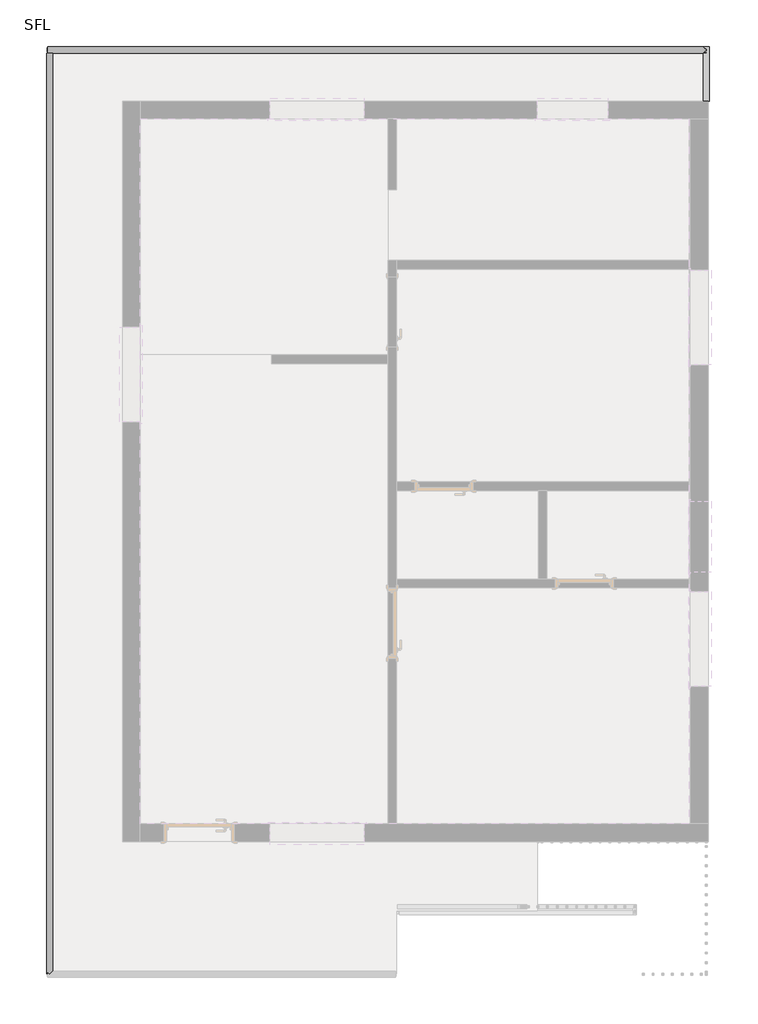
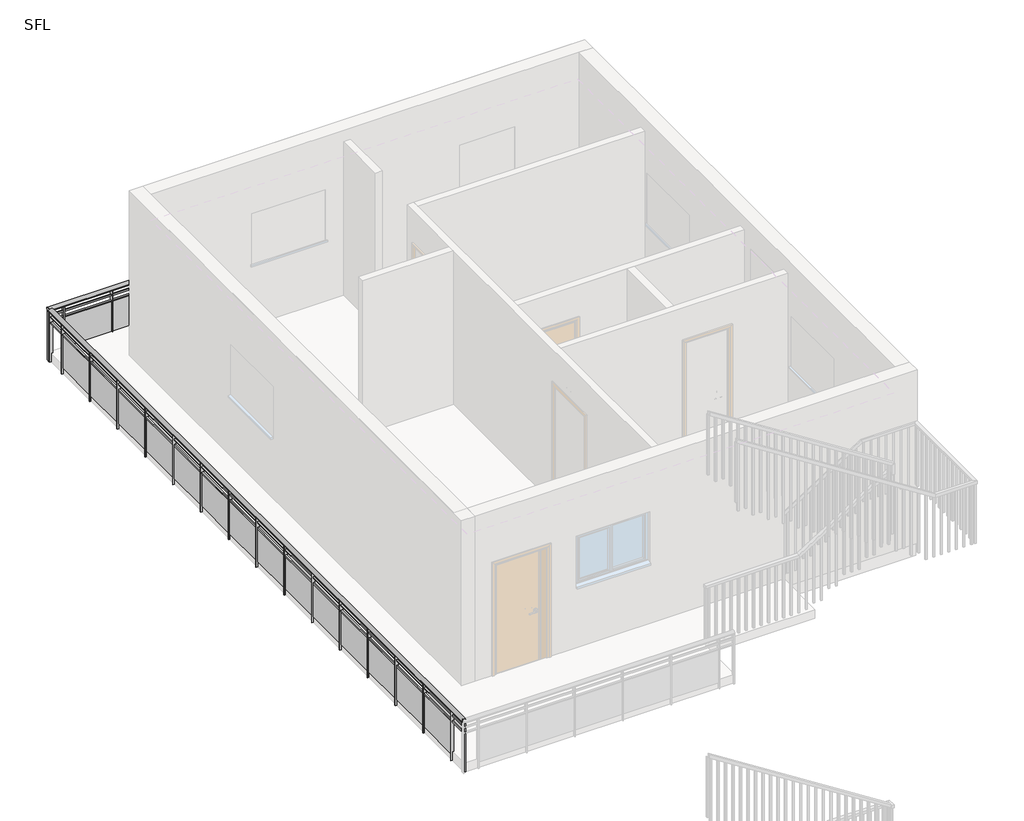
# One storey, part 4 of 4: 3 railings.
"""IFC4 building model written with IfcOpenShell, lengths in millimetres."""

from ifc_helpers import new_model, si_unit, point, frame, origin, place, context, project, spatial, polyline, ellipse_curve, trimmed, outline, extrude, element, save
from ifc_brep_helpers import plane_surface, extruded_surface, advanced_brep

model = new_model("IFC4")

# Units and contexts
model_context = context("Model", 3, world=origin())
ifc_project = project(units=[si_unit("LENGTHUNIT", "METRE", prefix="MILLI")], contexts=[model_context])

# Site, building, storey
site = spatial("IfcSite", under=ifc_project)
building = spatial("IfcBuilding", under=site)
storey = spatial("IfcBuildingStorey", under=building, Name="SFL", Elevation=6583.68)

# Railings
placement = place(None, origin())
element("IfcRailing", 1, ObjectType="Glass_Panel-Bottom_Fill", at=placement, inside=storey, context=model_context, shape_type="SolidModel", body=[
    advanced_brep(
    [(-15004.4132565, 42.847874, 7483.68), (-15004.4132565, -37.152126, 7483.68), (-6495.4132565, 42.847874, 7483.68), (-6495.4132565, -37.152126, 7483.68)],
    [
        (0, 1, ellipse_curve(frame((-15004.4132565, 2.847874, 7483.68), z_axis=(-1.0, 0.0, 0.0), x_axis=(0.0, -1.0, 0.0)), 40.0, 30.0)),
        (1, 0, ellipse_curve(frame((-15004.4132565, 2.847874, 7483.68), z_axis=(-1.0, 0.0, 0.0), x_axis=(0.0, -1.0, 0.0)), 40.0, 30.0)),
        (2, 3, ellipse_curve(frame((-6495.4132565, 2.847874, 7483.68), z_axis=(1.0, 0.0, 0.0), x_axis=(0.0, -1.0, 0.0)), 40.0, 30.0)),
        (3, 2, ellipse_curve(frame((-6495.4132565, 2.847874, 7483.68), z_axis=(1.0, 0.0, 0.0), x_axis=(0.0, -1.0, 0.0)), 40.0, 30.0)),
        (0, 2),
        (3, 1),
    ],
    [
        plane_surface(frame((-15004.4132565, 2.847874, 7483.68), z_axis=(-1.0, 0.0, 0.0), x_axis=(0.0, 1.0, 0.0))),
        plane_surface(frame((-6495.4132565, 2.847874, 7483.68), z_axis=(1.0, 0.0, 0.0), x_axis=(0.0, 1.0, 0.0))),
        extruded_surface(trimmed(ellipse_curve(frame((-6495.4132565, 2.847874, 7483.68), z_axis=(-1.0, 0.0, 0.0), x_axis=(0.0, -1.0, 0.0)), 40.0, 30.0), [point((-6495.4132565, 42.847874, 7483.68))], [point((-6495.4132565, -37.152126, 7483.68))], True, "CARTESIAN"), (-8509.0, 0.0, 0.0), 8509.0),
        extruded_surface(trimmed(ellipse_curve(frame((-6495.4132565, 2.847874, 7483.68), z_axis=(-1.0, 0.0, 0.0), x_axis=(0.0, -1.0, 0.0)), 40.0, 30.0), [point((-6495.4132565, -37.152126, 7483.68))], [point((-6495.4132565, 42.847874, 7483.68))], True, "CARTESIAN"), (-8509.0, 0.0, 0.0), 8509.0),
    ],
    [
        (0, [[1, 2]]),
        (1, [[3, 4]]),
        (2, [[-1, 5, -4, 6]]),
        (3, [[-2, -6, -3, -5]]),
    ],
),
    extrude(outline(polyline([(-15004.4132565, -6.5428911), (-15004.4132565, 13.4571089), (-6495.4132565, 13.4571089), (-6495.4132565, -6.5428911), (-15004.4132565, -6.5428911)])), frame((0.0, 0.0, 7363.68), z_axis=(0.0, 0.0, 1.0), x_axis=(1.0, 0.0, 0.0)), (0.0, 0.0, 1.0), 20.0),
    extrude(outline(polyline([(-15004.4132565, -6.5428911), (-15004.4132565, 13.4571089), (-6495.4132565, 13.4571089), (-6495.4132565, -6.5428911), (-15004.4132565, -6.5428911)])), frame((0.0, 0.0, 7263.68), z_axis=(0.0, 0.0, 1.0), x_axis=(1.0, 0.0, 0.0)), (0.0, 0.0, 1.0), 20.0),
    extrude(outline(polyline([(-6755.9132565, 28.4571089), (-6743.9132565, 28.4571089), (-6743.9132565, -21.5428911), (-6755.9132565, -21.5428911), (-6755.9132565, 28.4571089)])), frame((0.0, 0.0, 6583.68), z_axis=(0.0, 0.0, 1.0), x_axis=(1.0, 0.0, 0.0)), (0.0, 0.0, 1.0), 870.0),
    extrude(outline(polyline([(-7549.9132565, 1.7322988), (-6749.9132565, 1.7322988), (-6749.9132565, -3.2677012), (-7549.9132565, -3.2677012), (-7549.9132565, 1.7322988)])), frame((0.0, 0.0, 6683.68), z_axis=(0.0, 0.0, 1.0), x_axis=(1.0, 0.0, 0.0)), (0.0, 0.0, 1.0), 580.0),
    extrude(outline(polyline([(-7555.9132565, 28.4571089), (-7543.9132565, 28.4571089), (-7543.9132565, -21.5428911), (-7555.9132565, -21.5428911), (-7555.9132565, 28.4571089)])), frame((0.0, 0.0, 6583.68), z_axis=(0.0, 0.0, 1.0), x_axis=(1.0, 0.0, 0.0)), (0.0, 0.0, 1.0), 870.0),
    extrude(outline(polyline([(-8349.9132565, 1.7322988), (-7549.9132565, 1.7322988), (-7549.9132565, -3.2677012), (-8349.9132565, -3.2677012), (-8349.9132565, 1.7322988)])), frame((0.0, 0.0, 6683.68), z_axis=(0.0, 0.0, 1.0), x_axis=(1.0, 0.0, 0.0)), (0.0, 0.0, 1.0), 580.0),
    extrude(outline(polyline([(-8355.9132565, 28.4571089), (-8343.9132565, 28.4571089), (-8343.9132565, -21.5428911), (-8355.9132565, -21.5428911), (-8355.9132565, 28.4571089)])), frame((0.0, 0.0, 6583.68), z_axis=(0.0, 0.0, 1.0), x_axis=(1.0, 0.0, 0.0)), (0.0, 0.0, 1.0), 870.0),
    extrude(outline(polyline([(-9149.9132565, 1.7322988), (-8349.9132565, 1.7322988), (-8349.9132565, -3.2677012), (-9149.9132565, -3.2677012), (-9149.9132565, 1.7322988)])), frame((0.0, 0.0, 6683.68), z_axis=(0.0, 0.0, 1.0), x_axis=(1.0, 0.0, 0.0)), (0.0, 0.0, 1.0), 580.0),
    extrude(outline(polyline([(-9155.9132565, 28.4571089), (-9143.9132565, 28.4571089), (-9143.9132565, -21.5428911), (-9155.9132565, -21.5428911), (-9155.9132565, 28.4571089)])), frame((0.0, 0.0, 6583.68), z_axis=(0.0, 0.0, 1.0), x_axis=(1.0, 0.0, 0.0)), (0.0, 0.0, 1.0), 870.0),
    extrude(outline(polyline([(-9949.9132565, 1.7322988), (-9149.9132565, 1.7322988), (-9149.9132565, -3.2677012), (-9949.9132565, -3.2677012), (-9949.9132565, 1.7322988)])), frame((0.0, 0.0, 6683.68), z_axis=(0.0, 0.0, 1.0), x_axis=(1.0, 0.0, 0.0)), (0.0, 0.0, 1.0), 580.0),
    extrude(outline(polyline([(-9955.9132565, 28.4571089), (-9943.9132565, 28.4571089), (-9943.9132565, -21.5428911), (-9955.9132565, -21.5428911), (-9955.9132565, 28.4571089)])), frame((0.0, 0.0, 6583.68), z_axis=(0.0, 0.0, 1.0), x_axis=(1.0, 0.0, 0.0)), (0.0, 0.0, 1.0), 870.0),
    extrude(outline(polyline([(-10749.9132565, 1.7322988), (-9949.9132565, 1.7322988), (-9949.9132565, -3.2677012), (-10749.9132565, -3.2677012), (-10749.9132565, 1.7322988)])), frame((0.0, 0.0, 6683.68), z_axis=(0.0, 0.0, 1.0), x_axis=(1.0, 0.0, 0.0)), (0.0, 0.0, 1.0), 580.0),
    extrude(outline(polyline([(-10755.9132565, 28.4571089), (-10743.9132565, 28.4571089), (-10743.9132565, -21.5428911), (-10755.9132565, -21.5428911), (-10755.9132565, 28.4571089)])), frame((0.0, 0.0, 6583.68), z_axis=(0.0, 0.0, 1.0), x_axis=(1.0, 0.0, 0.0)), (0.0, 0.0, 1.0), 870.0),
    extrude(outline(polyline([(-11549.9132565, 1.7322988), (-10749.9132565, 1.7322988), (-10749.9132565, -3.2677012), (-11549.9132565, -3.2677012), (-11549.9132565, 1.7322988)])), frame((0.0, 0.0, 6683.68), z_axis=(0.0, 0.0, 1.0), x_axis=(1.0, 0.0, 0.0)), (0.0, 0.0, 1.0), 580.0),
    extrude(outline(polyline([(-11555.9132565, 28.4571089), (-11543.9132565, 28.4571089), (-11543.9132565, -21.5428911), (-11555.9132565, -21.5428911), (-11555.9132565, 28.4571089)])), frame((0.0, 0.0, 6583.68), z_axis=(0.0, 0.0, 1.0), x_axis=(1.0, 0.0, 0.0)), (0.0, 0.0, 1.0), 870.0),
    extrude(outline(polyline([(-12349.9132565, 1.7322988), (-11549.9132565, 1.7322988), (-11549.9132565, -3.2677012), (-12349.9132565, -3.2677012), (-12349.9132565, 1.7322988)])), frame((0.0, 0.0, 6683.68), z_axis=(0.0, 0.0, 1.0), x_axis=(1.0, 0.0, 0.0)), (0.0, 0.0, 1.0), 580.0),
    extrude(outline(polyline([(-12355.9132565, 28.4571089), (-12343.9132565, 28.4571089), (-12343.9132565, -21.5428911), (-12355.9132565, -21.5428911), (-12355.9132565, 28.4571089)])), frame((0.0, 0.0, 6583.68), z_axis=(0.0, 0.0, 1.0), x_axis=(1.0, 0.0, 0.0)), (0.0, 0.0, 1.0), 870.0),
    extrude(outline(polyline([(-13149.9132565, 1.7322988), (-12349.9132565, 1.7322988), (-12349.9132565, -3.2677012), (-13149.9132565, -3.2677012), (-13149.9132565, 1.7322988)])), frame((0.0, 0.0, 6683.68), z_axis=(0.0, 0.0, 1.0), x_axis=(1.0, 0.0, 0.0)), (0.0, 0.0, 1.0), 580.0),
    extrude(outline(polyline([(-13155.9132565, 28.4571089), (-13143.9132565, 28.4571089), (-13143.9132565, -21.5428911), (-13155.9132565, -21.5428911), (-13155.9132565, 28.4571089)])), frame((0.0, 0.0, 6583.68), z_axis=(0.0, 0.0, 1.0), x_axis=(1.0, 0.0, 0.0)), (0.0, 0.0, 1.0), 870.0),
    extrude(outline(polyline([(-13949.9132565, 1.7322988), (-13149.9132565, 1.7322988), (-13149.9132565, -3.2677012), (-13949.9132565, -3.2677012), (-13949.9132565, 1.7322988)])), frame((0.0, 0.0, 6683.68), z_axis=(0.0, 0.0, 1.0), x_axis=(1.0, 0.0, 0.0)), (0.0, 0.0, 1.0), 580.0),
    extrude(outline(polyline([(-13955.9132565, 28.4571089), (-13943.9132565, 28.4571089), (-13943.9132565, -21.5428911), (-13955.9132565, -21.5428911), (-13955.9132565, 28.4571089)])), frame((0.0, 0.0, 6583.68), z_axis=(0.0, 0.0, 1.0), x_axis=(1.0, 0.0, 0.0)), (0.0, 0.0, 1.0), 870.0),
    extrude(outline(polyline([(-14749.9132565, 1.7322988), (-13949.9132565, 1.7322988), (-13949.9132565, -3.2677012), (-14749.9132565, -3.2677012), (-14749.9132565, 1.7322988)])), frame((0.0, 0.0, 6683.68), z_axis=(0.0, 0.0, 1.0), x_axis=(1.0, 0.0, 0.0)), (0.0, 0.0, 1.0), 580.0),
    extrude(outline(polyline([(-14755.9132565, 28.4571089), (-14743.9132565, 28.4571089), (-14743.9132565, -21.5428911), (-14755.9132565, -21.5428911), (-14755.9132565, 28.4571089)])), frame((0.0, 0.0, 6583.68), z_axis=(0.0, 0.0, 1.0), x_axis=(1.0, 0.0, 0.0)), (0.0, 0.0, 1.0), 870.0),
    extrude(outline(polyline([(-6503.4132565, 28.4571089), (-6491.4132565, 28.4571089), (-6491.4132565, -21.5428911), (-6503.4132565, -21.5428911), (-6503.4132565, 28.4571089)])), frame((0.0, 0.0, 6583.68), z_axis=(0.0, 0.0, 1.0), x_axis=(1.0, 0.0, 0.0)), (0.0, 0.0, 1.0), 870.0),
    extrude(outline(polyline([(-15008.4132565, 28.4571089), (-14996.4132565, 28.4571089), (-14996.4132565, -21.5428911), (-15008.4132565, -21.5428911), (-15008.4132565, 28.4571089)])), frame((0.0, 0.0, 6583.68), z_axis=(0.0, 0.0, 1.0), x_axis=(1.0, 0.0, 0.0)), (0.0, 0.0, 1.0), 870.0),
])
element("IfcRailing", 2, ObjectType="Glass_Panel-Bottom_Fill", at=placement, inside=storey, context=model_context, shape_type="SolidModel", body=[
    advanced_brep(
    [(-14939.9512783, -37.152126, 7483.68), (-15019.9512783, -37.152126, 7483.68), (-14939.9512783, -11928.1928911, 7483.68), (-15019.9512783, -11928.1928911, 7483.68)],
    [
        (0, 1, ellipse_curve(frame((-14979.9512783, -37.152126, 7483.68), z_axis=(0.0, 1.0, 0.0), x_axis=(-1.0, 0.0, 0.0)), 40.0, 30.0)),
        (1, 0, ellipse_curve(frame((-14979.9512783, -37.152126, 7483.68), z_axis=(0.0, 1.0, 0.0), x_axis=(-1.0, 0.0, 0.0)), 40.0, 30.0)),
        (2, 3, ellipse_curve(frame((-14979.9512783, -11928.1928911, 7483.68), z_axis=(0.0, -1.0, 0.0), x_axis=(-1.0, 0.0, 0.0)), 40.0, 30.0)),
        (3, 2, ellipse_curve(frame((-14979.9512783, -11928.1928911, 7483.68), z_axis=(0.0, -1.0, 0.0), x_axis=(-1.0, 0.0, 0.0)), 40.0, 30.0)),
        (0, 2),
        (3, 1),
    ],
    [
        plane_surface(frame((-14979.9512783, -37.152126, 7483.68), z_axis=(0.0, 1.0, 0.0), x_axis=(0.0, 0.0, -1.0))),
        plane_surface(frame((-14979.9512783, -11928.1928911, 7483.68), z_axis=(0.0, -1.0, 0.0), x_axis=(0.0, 0.0, -1.0))),
        extruded_surface(trimmed(ellipse_curve(frame((-14979.9512783, -11928.1928911, 7483.68), z_axis=(0.0, 1.0, 0.0), x_axis=(-1.0, 0.0, 0.0)), 40.0, 30.0), [point((-14939.9512783, -11928.1928911, 7483.68))], [point((-15019.9512783, -11928.1928911, 7483.68))], True, "CARTESIAN"), (0.0, 11891.040765099999, 0.0), 11891.040765099999),
        extruded_surface(trimmed(ellipse_curve(frame((-14979.9512783, -11928.1928911, 7483.68), z_axis=(0.0, 1.0, 0.0), x_axis=(-1.0, 0.0, 0.0)), 40.0, 30.0), [point((-15019.9512783, -11928.1928911, 7483.68))], [point((-14939.9512783, -11928.1928911, 7483.68))], True, "CARTESIAN"), (0.0, 11891.040765099999, 0.0), 11891.040765099999),
    ],
    [
        (0, [[1, 2]]),
        (1, [[3, 4]]),
        (2, [[-1, 5, -4, 6]]),
        (3, [[-2, -6, -3, -5]]),
    ],
),
    extrude(outline(polyline([(-14989.3420435, -37.152126), (-14969.3420435, -37.152126), (-14969.3420435, -11928.1928911), (-14989.3420435, -11928.1928911), (-14989.3420435, -37.152126)])), frame((0.0, 0.0, 7363.68), z_axis=(0.0, 0.0, 1.0), x_axis=(1.0, 0.0, 0.0)), (0.0, 0.0, 1.0), 20.0),
    extrude(outline(polyline([(-14989.3420435, -37.152126), (-14969.3420435, -37.152126), (-14969.3420435, -11928.1928911), (-14989.3420435, -11928.1928911), (-14989.3420435, -37.152126)])), frame((0.0, 0.0, 7263.68), z_axis=(0.0, 0.0, 1.0), x_axis=(1.0, 0.0, 0.0)), (0.0, 0.0, 1.0), 20.0),
    extrude(outline(polyline([(-14954.3420435, -11576.6725086), (-14954.3420435, -11588.6725086), (-15004.3420435, -11588.6725086), (-15004.3420435, -11576.6725086), (-14954.3420435, -11576.6725086)])), frame((0.0, 0.0, 6583.68), z_axis=(0.0, 0.0, 1.0), x_axis=(1.0, 0.0, 0.0)), (0.0, 0.0, 1.0), 870.0),
    extrude(outline(polyline([(-14981.0668536, -10782.6725086), (-14981.0668536, -11582.6725086), (-14986.0668536, -11582.6725086), (-14986.0668536, -10782.6725086), (-14981.0668536, -10782.6725086)])), frame((0.0, 0.0, 6683.68), z_axis=(0.0, 0.0, 1.0), x_axis=(1.0, 0.0, 0.0)), (0.0, 0.0, 1.0), 580.0),
    extrude(outline(polyline([(-14954.3420435, -10776.6725086), (-14954.3420435, -10788.6725086), (-15004.3420435, -10788.6725086), (-15004.3420435, -10776.6725086), (-14954.3420435, -10776.6725086)])), frame((0.0, 0.0, 6583.68), z_axis=(0.0, 0.0, 1.0), x_axis=(1.0, 0.0, 0.0)), (0.0, 0.0, 1.0), 870.0),
    extrude(outline(polyline([(-14981.0668536, -9982.6725086), (-14981.0668536, -10782.6725086), (-14986.0668536, -10782.6725086), (-14986.0668536, -9982.6725086), (-14981.0668536, -9982.6725086)])), frame((0.0, 0.0, 6683.68), z_axis=(0.0, 0.0, 1.0), x_axis=(1.0, 0.0, 0.0)), (0.0, 0.0, 1.0), 580.0),
    extrude(outline(polyline([(-14954.3420435, -9976.6725086), (-14954.3420435, -9988.6725086), (-15004.3420435, -9988.6725086), (-15004.3420435, -9976.6725086), (-14954.3420435, -9976.6725086)])), frame((0.0, 0.0, 6583.68), z_axis=(0.0, 0.0, 1.0), x_axis=(1.0, 0.0, 0.0)), (0.0, 0.0, 1.0), 870.0),
    extrude(outline(polyline([(-14981.0668536, -9182.6725086), (-14981.0668536, -9982.6725086), (-14986.0668536, -9982.6725086), (-14986.0668536, -9182.6725086), (-14981.0668536, -9182.6725086)])), frame((0.0, 0.0, 6683.68), z_axis=(0.0, 0.0, 1.0), x_axis=(1.0, 0.0, 0.0)), (0.0, 0.0, 1.0), 580.0),
    extrude(outline(polyline([(-14954.3420435, -9176.6725086), (-14954.3420435, -9188.6725086), (-15004.3420435, -9188.6725086), (-15004.3420435, -9176.6725086), (-14954.3420435, -9176.6725086)])), frame((0.0, 0.0, 6583.68), z_axis=(0.0, 0.0, 1.0), x_axis=(1.0, 0.0, 0.0)), (0.0, 0.0, 1.0), 870.0),
    extrude(outline(polyline([(-14981.0668536, -8382.6725086), (-14981.0668536, -9182.6725086), (-14986.0668536, -9182.6725086), (-14986.0668536, -8382.6725086), (-14981.0668536, -8382.6725086)])), frame((0.0, 0.0, 6683.68), z_axis=(0.0, 0.0, 1.0), x_axis=(1.0, 0.0, 0.0)), (0.0, 0.0, 1.0), 580.0),
    extrude(outline(polyline([(-14954.3420435, -8376.6725086), (-14954.3420435, -8388.6725086), (-15004.3420435, -8388.6725086), (-15004.3420435, -8376.6725086), (-14954.3420435, -8376.6725086)])), frame((0.0, 0.0, 6583.68), z_axis=(0.0, 0.0, 1.0), x_axis=(1.0, 0.0, 0.0)), (0.0, 0.0, 1.0), 870.0),
    extrude(outline(polyline([(-14981.0668536, -7582.6725086), (-14981.0668536, -8382.6725086), (-14986.0668536, -8382.6725086), (-14986.0668536, -7582.6725086), (-14981.0668536, -7582.6725086)])), frame((0.0, 0.0, 6683.68), z_axis=(0.0, 0.0, 1.0), x_axis=(1.0, 0.0, 0.0)), (0.0, 0.0, 1.0), 580.0),
    extrude(outline(polyline([(-14954.3420435, -7576.6725086), (-14954.3420435, -7588.6725086), (-15004.3420435, -7588.6725086), (-15004.3420435, -7576.6725086), (-14954.3420435, -7576.6725086)])), frame((0.0, 0.0, 6583.68), z_axis=(0.0, 0.0, 1.0), x_axis=(1.0, 0.0, 0.0)), (0.0, 0.0, 1.0), 870.0),
    extrude(outline(polyline([(-14981.0668536, -6782.6725086), (-14981.0668536, -7582.6725086), (-14986.0668536, -7582.6725086), (-14986.0668536, -6782.6725086), (-14981.0668536, -6782.6725086)])), frame((0.0, 0.0, 6683.68), z_axis=(0.0, 0.0, 1.0), x_axis=(1.0, 0.0, 0.0)), (0.0, 0.0, 1.0), 580.0),
    extrude(outline(polyline([(-14954.3420435, -6776.6725086), (-14954.3420435, -6788.6725086), (-15004.3420435, -6788.6725086), (-15004.3420435, -6776.6725086), (-14954.3420435, -6776.6725086)])), frame((0.0, 0.0, 6583.68), z_axis=(0.0, 0.0, 1.0), x_axis=(1.0, 0.0, 0.0)), (0.0, 0.0, 1.0), 870.0),
    extrude(outline(polyline([(-14981.0668536, -5982.6725086), (-14981.0668536, -6782.6725086), (-14986.0668536, -6782.6725086), (-14986.0668536, -5982.6725086), (-14981.0668536, -5982.6725086)])), frame((0.0, 0.0, 6683.68), z_axis=(0.0, 0.0, 1.0), x_axis=(1.0, 0.0, 0.0)), (0.0, 0.0, 1.0), 580.0),
    extrude(outline(polyline([(-14954.3420435, -5976.6725086), (-14954.3420435, -5988.6725086), (-15004.3420435, -5988.6725086), (-15004.3420435, -5976.6725086), (-14954.3420435, -5976.6725086)])), frame((0.0, 0.0, 6583.68), z_axis=(0.0, 0.0, 1.0), x_axis=(1.0, 0.0, 0.0)), (0.0, 0.0, 1.0), 870.0),
    extrude(outline(polyline([(-14981.0668536, -5182.6725086), (-14981.0668536, -5982.6725086), (-14986.0668536, -5982.6725086), (-14986.0668536, -5182.6725086), (-14981.0668536, -5182.6725086)])), frame((0.0, 0.0, 6683.68), z_axis=(0.0, 0.0, 1.0), x_axis=(1.0, 0.0, 0.0)), (0.0, 0.0, 1.0), 580.0),
    extrude(outline(polyline([(-14954.3420435, -5176.6725086), (-14954.3420435, -5188.6725086), (-15004.3420435, -5188.6725086), (-15004.3420435, -5176.6725086), (-14954.3420435, -5176.6725086)])), frame((0.0, 0.0, 6583.68), z_axis=(0.0, 0.0, 1.0), x_axis=(1.0, 0.0, 0.0)), (0.0, 0.0, 1.0), 870.0),
    extrude(outline(polyline([(-14981.0668536, -4382.6725086), (-14981.0668536, -5182.6725086), (-14986.0668536, -5182.6725086), (-14986.0668536, -4382.6725086), (-14981.0668536, -4382.6725086)])), frame((0.0, 0.0, 6683.68), z_axis=(0.0, 0.0, 1.0), x_axis=(1.0, 0.0, 0.0)), (0.0, 0.0, 1.0), 580.0),
    extrude(outline(polyline([(-14954.3420435, -4376.6725086), (-14954.3420435, -4388.6725086), (-15004.3420435, -4388.6725086), (-15004.3420435, -4376.6725086), (-14954.3420435, -4376.6725086)])), frame((0.0, 0.0, 6583.68), z_axis=(0.0, 0.0, 1.0), x_axis=(1.0, 0.0, 0.0)), (0.0, 0.0, 1.0), 870.0),
    extrude(outline(polyline([(-14981.0668536, -3582.6725086), (-14981.0668536, -4382.6725086), (-14986.0668536, -4382.6725086), (-14986.0668536, -3582.6725086), (-14981.0668536, -3582.6725086)])), frame((0.0, 0.0, 6683.68), z_axis=(0.0, 0.0, 1.0), x_axis=(1.0, 0.0, 0.0)), (0.0, 0.0, 1.0), 580.0),
    extrude(outline(polyline([(-14954.3420435, -3576.6725086), (-14954.3420435, -3588.6725086), (-15004.3420435, -3588.6725086), (-15004.3420435, -3576.6725086), (-14954.3420435, -3576.6725086)])), frame((0.0, 0.0, 6583.68), z_axis=(0.0, 0.0, 1.0), x_axis=(1.0, 0.0, 0.0)), (0.0, 0.0, 1.0), 870.0),
    extrude(outline(polyline([(-14981.0668536, -2782.6725086), (-14981.0668536, -3582.6725086), (-14986.0668536, -3582.6725086), (-14986.0668536, -2782.6725086), (-14981.0668536, -2782.6725086)])), frame((0.0, 0.0, 6683.68), z_axis=(0.0, 0.0, 1.0), x_axis=(1.0, 0.0, 0.0)), (0.0, 0.0, 1.0), 580.0),
    extrude(outline(polyline([(-14954.3420435, -2776.6725086), (-14954.3420435, -2788.6725086), (-15004.3420435, -2788.6725086), (-15004.3420435, -2776.6725086), (-14954.3420435, -2776.6725086)])), frame((0.0, 0.0, 6583.68), z_axis=(0.0, 0.0, 1.0), x_axis=(1.0, 0.0, 0.0)), (0.0, 0.0, 1.0), 870.0),
    extrude(outline(polyline([(-14981.0668536, -1982.6725086), (-14981.0668536, -2782.6725086), (-14986.0668536, -2782.6725086), (-14986.0668536, -1982.6725086), (-14981.0668536, -1982.6725086)])), frame((0.0, 0.0, 6683.68), z_axis=(0.0, 0.0, 1.0), x_axis=(1.0, 0.0, 0.0)), (0.0, 0.0, 1.0), 580.0),
    extrude(outline(polyline([(-14954.3420435, -1976.6725086), (-14954.3420435, -1988.6725086), (-15004.3420435, -1988.6725086), (-15004.3420435, -1976.6725086), (-14954.3420435, -1976.6725086)])), frame((0.0, 0.0, 6583.68), z_axis=(0.0, 0.0, 1.0), x_axis=(1.0, 0.0, 0.0)), (0.0, 0.0, 1.0), 870.0),
    extrude(outline(polyline([(-14981.0668536, -1182.6725086), (-14981.0668536, -1982.6725086), (-14986.0668536, -1982.6725086), (-14986.0668536, -1182.6725086), (-14981.0668536, -1182.6725086)])), frame((0.0, 0.0, 6683.68), z_axis=(0.0, 0.0, 1.0), x_axis=(1.0, 0.0, 0.0)), (0.0, 0.0, 1.0), 580.0),
    extrude(outline(polyline([(-14954.3420435, -1176.6725086), (-14954.3420435, -1188.6725086), (-15004.3420435, -1188.6725086), (-15004.3420435, -1176.6725086), (-14954.3420435, -1176.6725086)])), frame((0.0, 0.0, 6583.68), z_axis=(0.0, 0.0, 1.0), x_axis=(1.0, 0.0, 0.0)), (0.0, 0.0, 1.0), 870.0),
    extrude(outline(polyline([(-14981.0668536, -382.6725086), (-14981.0668536, -1182.6725086), (-14986.0668536, -1182.6725086), (-14986.0668536, -382.6725086), (-14981.0668536, -382.6725086)])), frame((0.0, 0.0, 6683.68), z_axis=(0.0, 0.0, 1.0), x_axis=(1.0, 0.0, 0.0)), (0.0, 0.0, 1.0), 580.0),
    extrude(outline(polyline([(-14954.3420435, -376.6725086), (-14954.3420435, -388.6725086), (-15004.3420435, -388.6725086), (-15004.3420435, -376.6725086), (-14954.3420435, -376.6725086)])), frame((0.0, 0.0, 6583.68), z_axis=(0.0, 0.0, 1.0), x_axis=(1.0, 0.0, 0.0)), (0.0, 0.0, 1.0), 870.0),
    extrude(outline(polyline([(-14954.3420435, -11920.1928911), (-14954.3420435, -11932.1928911), (-15004.3420435, -11932.1928911), (-15004.3420435, -11920.1928911), (-14954.3420435, -11920.1928911)])), frame((0.0, 0.0, 6583.68), z_axis=(0.0, 0.0, 1.0), x_axis=(1.0, 0.0, 0.0)), (0.0, 0.0, 1.0), 870.0),
    extrude(outline(polyline([(-14954.3420435, -33.152126), (-14954.3420435, -45.152126), (-15004.3420435, -45.152126), (-15004.3420435, -33.152126), (-14954.3420435, -33.152126)])), frame((0.0, 0.0, 6583.68), z_axis=(0.0, 0.0, 1.0), x_axis=(1.0, 0.0, 0.0)), (0.0, 0.0, 1.0), 870.0),
])
element("IfcRailing", 3, ObjectType="Glass_Panel-Bottom_Fill", at=placement, inside=storey, context=model_context, shape_type="SolidModel", body=[
    advanced_brep(
    [(-6534.8040217, -656.9593981, 7483.68), (-6454.8040217, -656.9593981, 7483.68), (-6534.8040217, 42.847874, 7483.68), (-6454.8040217, 42.847874, 7483.68)],
    [
        (0, 1, ellipse_curve(frame((-6494.8040217, -656.9593981, 7483.68), z_axis=(0.0, -1.0, 0.0), x_axis=(1.0, 0.0, 0.0)), 40.0, 30.0)),
        (1, 0, ellipse_curve(frame((-6494.8040217, -656.9593981, 7483.68), z_axis=(0.0, -1.0, 0.0), x_axis=(1.0, 0.0, 0.0)), 40.0, 30.0)),
        (2, 3, ellipse_curve(frame((-6494.8040217, 42.847874, 7483.68), z_axis=(0.0, 1.0, 0.0), x_axis=(1.0, 0.0, 0.0)), 40.0, 30.0)),
        (3, 2, ellipse_curve(frame((-6494.8040217, 42.847874, 7483.68), z_axis=(0.0, 1.0, 0.0), x_axis=(1.0, 0.0, 0.0)), 40.0, 30.0)),
        (0, 2),
        (3, 1),
    ],
    [
        plane_surface(frame((-6494.8040217, -656.9593981, 7483.68), z_axis=(0.0, -1.0, 0.0), x_axis=(0.0, 0.0, 1.0))),
        plane_surface(frame((-6494.8040217, 42.847874, 7483.68), z_axis=(0.0, 1.0, 0.0), x_axis=(0.0, 0.0, 1.0))),
        extruded_surface(trimmed(ellipse_curve(frame((-6494.8040217, 42.847874, 7483.68), z_axis=(0.0, -1.0, 0.0), x_axis=(1.0, 0.0, 0.0)), 40.0, 30.0), [point((-6534.8040217, 42.847874, 7483.68))], [point((-6454.8040217, 42.847874, 7483.68))], True, "CARTESIAN"), (0.0, -699.8072721000001, 0.0), 699.8072721000001),
        extruded_surface(trimmed(ellipse_curve(frame((-6494.8040217, 42.847874, 7483.68), z_axis=(0.0, -1.0, 0.0), x_axis=(1.0, 0.0, 0.0)), 40.0, 30.0), [point((-6454.8040217, 42.847874, 7483.68))], [point((-6534.8040217, 42.847874, 7483.68))], True, "CARTESIAN"), (0.0, -699.8072721000001, 0.0), 699.8072721000001),
    ],
    [
        (0, [[1, 2]]),
        (1, [[3, 4]]),
        (2, [[-1, 5, -4, 6]]),
        (3, [[-2, -6, -3, -5]]),
    ],
),
    extrude(outline(polyline([(-6485.4132565, -656.9593981), (-6505.4132565, -656.9593981), (-6505.4132565, 42.847874), (-6485.4132565, 42.847874), (-6485.4132565, -656.9593981)])), frame((0.0, 0.0, 7363.68), z_axis=(0.0, 0.0, 1.0), x_axis=(1.0, 0.0, 0.0)), (0.0, 0.0, 1.0), 20.0),
    extrude(outline(polyline([(-6485.4132565, -656.9593981), (-6505.4132565, -656.9593981), (-6505.4132565, 42.847874), (-6485.4132565, 42.847874), (-6485.4132565, -656.9593981)])), frame((0.0, 0.0, 7263.68), z_axis=(0.0, 0.0, 1.0), x_axis=(1.0, 0.0, 0.0)), (0.0, 0.0, 1.0), 20.0),
    extrude(outline(polyline([(-6520.4132565, 34.847874), (-6520.4132565, 46.847874), (-6470.4132565, 46.847874), (-6470.4132565, 34.847874), (-6520.4132565, 34.847874)])), frame((0.0, 0.0, 6583.68), z_axis=(0.0, 0.0, 1.0), x_axis=(1.0, 0.0, 0.0)), (0.0, 0.0, 1.0), 870.0),
    extrude(outline(polyline([(-6520.4132565, -660.9593981), (-6520.4132565, -648.9593981), (-6470.4132565, -648.9593981), (-6470.4132565, -660.9593981), (-6520.4132565, -660.9593981)])), frame((0.0, 0.0, 6583.68), z_axis=(0.0, 0.0, 1.0), x_axis=(1.0, 0.0, 0.0)), (0.0, 0.0, 1.0), 870.0),
])

save(model, "model.ifc")

# Revit data of these elements
# Type "Glass_Panel-Bottom_Fill"
#   built-in parameter 1008612 = 0.019685 (stored number, unit not read)
#   built-in parameter 1008611 = 0.019685 (stored number, unit not read)
#   built-in parameter 1008609 = 0.902231 (stored number, unit not read)
#   built-in parameter 1008604 = 0.19685 (stored number, unit not read)
#   built-in parameter 1008603 = 0.164042 (stored number, unit not read)
#   Railing Height = 2.952756 ft
#   built-in parameter 1008630 = 2
#   built-in parameter 1008610 = 2
# Elements 1, 2 (IfcRailing, "Glass_Panel-Bottom_Fill")
#   Phase Created = New Construction
#   Materials on its faces: "Metal - Stainless Steel,Polished", "Glass"
# Element 3 (IfcRailing, "Glass_Panel-Bottom_Fill")
#   Phase Created = New Construction
#   Materials on its faces: "Metal - Stainless Steel,Polished"
# Materials
#   "Metal - Stainless Steel,Polished": class "Metal", colour RGB 236 239 239, transparency 0, Cost = 0
#   "Glass": class "Glass", colour RGB 0 128 192, transparency 0.9, Description = "Soda Lime Glass", Cost = 0
